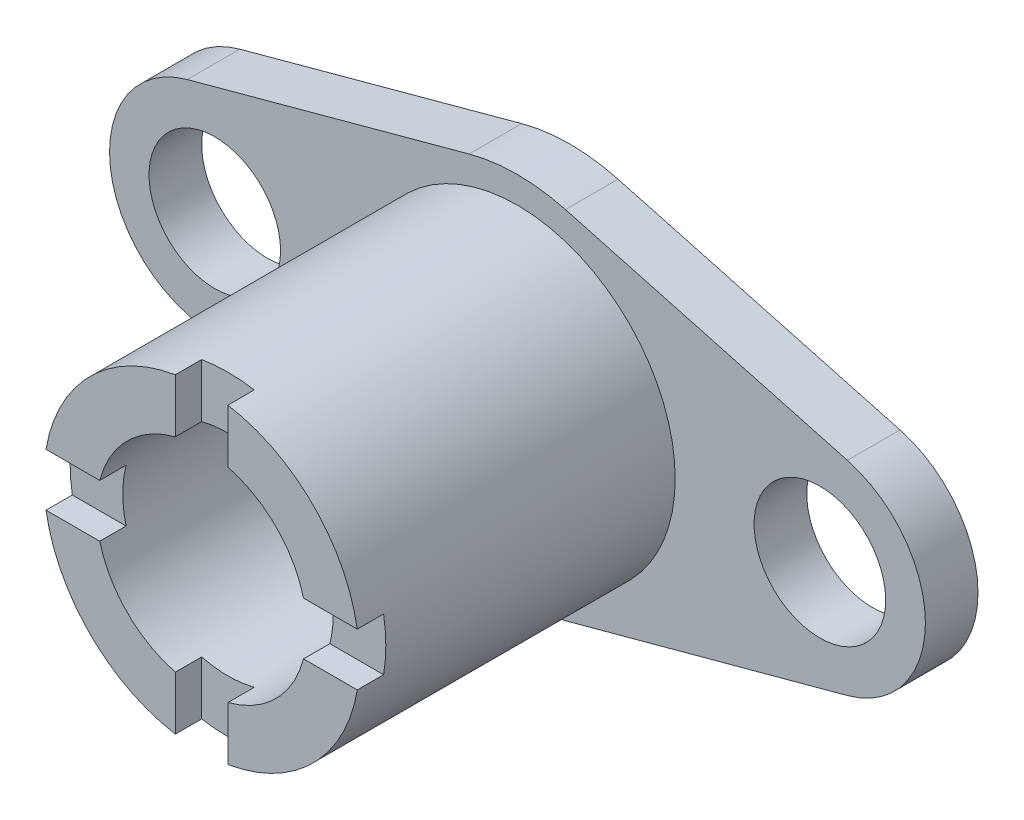
ISO-10303-21;
HEADER;
FILE_DESCRIPTION(('STEP AP214'),'2;1');
FILE_NAME('part.step','',(''),(''),'','','');
FILE_SCHEMA(('AUTOMOTIVE_DESIGN { 1 0 10303 214 1 1 1 1 }'));
ENDSEC;
DATA;
#1=APPLICATION_CONTEXT('core data for automotive mechanical design processes');
#2=APPLICATION_PROTOCOL_DEFINITION('international standard','automotive_design',2000,#1);
#3=PRODUCT_CONTEXT('',#1,'mechanical');
#4=PRODUCT('Part','Part','',(#3));
#5=PRODUCT_RELATED_PRODUCT_CATEGORY('part','',(#4));
#6=PRODUCT_DEFINITION_FORMATION('','',#4);
#7=PRODUCT_DEFINITION_CONTEXT('part definition',#1,'design');
#8=PRODUCT_DEFINITION('design','',#6,#7);
#9=PRODUCT_DEFINITION_SHAPE('','',#8);
#10=(LENGTH_UNIT() NAMED_UNIT(*) SI_UNIT(.MILLI.,.METRE.));
#11=(NAMED_UNIT(*) PLANE_ANGLE_UNIT() SI_UNIT($,.RADIAN.));
#12=(NAMED_UNIT(*) SI_UNIT($,.STERADIAN.) SOLID_ANGLE_UNIT());
#13=UNCERTAINTY_MEASURE_WITH_UNIT(LENGTH_MEASURE(1.E-05),#10,'distance_accuracy_value','');
#14=(GEOMETRIC_REPRESENTATION_CONTEXT(3) GLOBAL_UNCERTAINTY_ASSIGNED_CONTEXT((#13)) GLOBAL_UNIT_ASSIGNED_CONTEXT((#10,
#11,#12)) REPRESENTATION_CONTEXT('',''));
#15=CARTESIAN_POINT('',(0.,0.,0.));
#16=DIRECTION('',(0.,0.,1.));
#17=DIRECTION('',(1.,0.,0.));
#18=AXIS2_PLACEMENT_3D('',#15,#16,#17);
#19=CARTESIAN_POINT('',(0.,0.,70.));
#20=DIRECTION('',(0.,0.,-1.));
#21=DIRECTION('',(-1.,0.,0.));
#22=AXIS2_PLACEMENT_3D('',#19,#20,#21);
#23=CYLINDRICAL_SURFACE('',#22,30.);
#24=CARTESIAN_POINT('',(0.,0.,70.));
#25=DIRECTION('',(0.,0.,1.));
#26=DIRECTION('',(1.,0.,0.));
#27=AXIS2_PLACEMENT_3D('',#24,#25,#26);
#28=CIRCLE('',#27,30.);
#29=CARTESIAN_POINT('',(-29.5803989154981,-5.,70.));
#30=VERTEX_POINT('',#29);
#31=CARTESIAN_POINT('',(-5.,-29.5803989154981,70.));
#32=VERTEX_POINT('',#31);
#33=EDGE_CURVE('E751',#30,#32,#28,.T.);
#34=ORIENTED_EDGE('',*,*,#33,.F.);
#35=DIRECTION('',(0.,0.,1.));
#36=VECTOR('',#35,1.);
#37=CARTESIAN_POINT('',(-29.5803989154981,-5.,65.));
#38=LINE('',#37,#36);
#39=CARTESIAN_POINT('',(-29.5803989154981,-5.,65.));
#40=VERTEX_POINT('',#39);
#41=EDGE_CURVE('E233',#40,#30,#38,.T.);
#42=ORIENTED_EDGE('',*,*,#41,.F.);
#43=CARTESIAN_POINT('',(0.,0.,65.));
#44=DIRECTION('',(0.,0.,1.));
#45=DIRECTION('',(1.,0.,0.));
#46=AXIS2_PLACEMENT_3D('',#43,#44,#45);
#47=CIRCLE('',#46,30.);
#48=CARTESIAN_POINT('',(-29.5803989154981,5.,65.));
#49=VERTEX_POINT('',#48);
#50=EDGE_CURVE('E216',#49,#40,#47,.T.);
#51=ORIENTED_EDGE('',*,*,#50,.F.);
#52=DIRECTION('',(0.,0.,1.));
#53=VECTOR('',#52,1.);
#54=CARTESIAN_POINT('',(-29.5803989154981,5.,65.));
#55=LINE('',#54,#53);
#56=CARTESIAN_POINT('',(-29.5803989154981,5.,70.));
#57=VERTEX_POINT('',#56);
#58=EDGE_CURVE('E211',#49,#57,#55,.T.);
#59=ORIENTED_EDGE('',*,*,#58,.T.);
#60=CARTESIAN_POINT('',(-5.,29.5803989154981,70.));
#61=VERTEX_POINT('',#60);
#62=EDGE_CURVE('E324',#61,#57,#28,.T.);
#63=ORIENTED_EDGE('',*,*,#62,.F.);
#64=DIRECTION('',(0.,0.,1.));
#65=VECTOR('',#64,1.);
#66=CARTESIAN_POINT('',(-5.,29.5803989154981,65.));
#67=LINE('',#66,#65);
#68=CARTESIAN_POINT('',(-5.,29.5803989154981,65.));
#69=VERTEX_POINT('',#68);
#70=EDGE_CURVE('E257',#69,#61,#67,.T.);
#71=ORIENTED_EDGE('',*,*,#70,.F.);
#72=CARTESIAN_POINT('',(0.,0.,65.));
#73=DIRECTION('',(0.,0.,1.));
#74=DIRECTION('',(1.,0.,0.));
#75=AXIS2_PLACEMENT_3D('',#72,#73,#74);
#76=CIRCLE('',#75,30.);
#77=CARTESIAN_POINT('',(5.,29.5803989154981,65.));
#78=VERTEX_POINT('',#77);
#79=EDGE_CURVE('E238',#78,#69,#76,.T.);
#80=ORIENTED_EDGE('',*,*,#79,.F.);
#81=DIRECTION('',(0.,0.,1.));
#82=VECTOR('',#81,1.);
#83=CARTESIAN_POINT('',(5.,29.5803989154981,65.));
#84=LINE('',#83,#82);
#85=CARTESIAN_POINT('',(5.,29.5803989154981,70.));
#86=VERTEX_POINT('',#85);
#87=EDGE_CURVE('E242',#78,#86,#84,.T.);
#88=ORIENTED_EDGE('',*,*,#87,.T.);
#89=CARTESIAN_POINT('',(29.5803989154981,5.,70.));
#90=VERTEX_POINT('',#89);
#91=EDGE_CURVE('E316',#90,#86,#28,.T.);
#92=ORIENTED_EDGE('',*,*,#91,.F.);
#93=DIRECTION('',(0.,0.,1.));
#94=VECTOR('',#93,1.);
#95=CARTESIAN_POINT('',(29.5803989154981,5.,65.));
#96=LINE('',#95,#94);
#97=CARTESIAN_POINT('',(29.5803989154981,5.,65.));
#98=VERTEX_POINT('',#97);
#99=EDGE_CURVE('E310',#98,#90,#96,.T.);
#100=ORIENTED_EDGE('',*,*,#99,.F.);
#101=CARTESIAN_POINT('',(0.,0.,65.));
#102=DIRECTION('',(0.,0.,1.));
#103=DIRECTION('',(1.,0.,0.));
#104=AXIS2_PLACEMENT_3D('',#101,#102,#103);
#105=CIRCLE('',#104,30.);
#106=CARTESIAN_POINT('',(29.5803989154981,-5.,65.));
#107=VERTEX_POINT('',#106);
#108=EDGE_CURVE('E290',#107,#98,#105,.T.);
#109=ORIENTED_EDGE('',*,*,#108,.F.);
#110=DIRECTION('',(0.,0.,1.));
#111=VECTOR('',#110,1.);
#112=CARTESIAN_POINT('',(29.5803989154981,-5.,65.));
#113=LINE('',#112,#111);
#114=CARTESIAN_POINT('',(29.5803989154981,-5.,70.));
#115=VERTEX_POINT('',#114);
#116=EDGE_CURVE('E298',#107,#115,#113,.T.);
#117=ORIENTED_EDGE('',*,*,#116,.T.);
#118=CARTESIAN_POINT('',(5.,-29.5803989154981,70.));
#119=VERTEX_POINT('',#118);
#120=EDGE_CURVE('E321',#119,#115,#28,.T.);
#121=ORIENTED_EDGE('',*,*,#120,.F.);
#122=DIRECTION('',(0.,0.,1.));
#123=VECTOR('',#122,1.);
#124=CARTESIAN_POINT('',(5.,-29.5803989154981,65.));
#125=LINE('',#124,#123);
#126=CARTESIAN_POINT('',(5.,-29.5803989154981,65.));
#127=VERTEX_POINT('',#126);
#128=EDGE_CURVE('E272',#127,#119,#125,.T.);
#129=ORIENTED_EDGE('',*,*,#128,.F.);
#130=CARTESIAN_POINT('',(0.,0.,65.));
#131=DIRECTION('',(0.,0.,1.));
#132=DIRECTION('',(1.,0.,0.));
#133=AXIS2_PLACEMENT_3D('',#130,#131,#132);
#134=CIRCLE('',#133,30.);
#135=CARTESIAN_POINT('',(-5.,-29.5803989154981,65.));
#136=VERTEX_POINT('',#135);
#137=EDGE_CURVE('E258',#136,#127,#134,.T.);
#138=ORIENTED_EDGE('',*,*,#137,.F.);
#139=DIRECTION('',(0.,0.,1.));
#140=VECTOR('',#139,1.);
#141=CARTESIAN_POINT('',(-5.,-29.5803989154981,65.));
#142=LINE('',#141,#140);
#143=EDGE_CURVE('E247',#136,#32,#142,.T.);
#144=ORIENTED_EDGE('',*,*,#143,.T.);
#145=EDGE_LOOP('',(#34,#42,#51,#59,#63,#71,#80,#88,#92,#100,#109,#117,#121,#129,#138,#144));
#146=FACE_BOUND('',#145,.T.);
#147=CARTESIAN_POINT('',(0.,0.,10.));
#148=DIRECTION('',(0.,0.,1.));
#149=DIRECTION('',(1.,0.,0.));
#150=AXIS2_PLACEMENT_3D('',#147,#148,#149);
#151=CIRCLE('',#150,30.);
#152=CARTESIAN_POINT('',(30.,0.,10.));
#153=VERTEX_POINT('',#152);
#154=EDGE_CURVE('E313',#153,#153,#151,.T.);
#155=ORIENTED_EDGE('',*,*,#154,.T.);
#156=EDGE_LOOP('',(#155));
#157=FACE_BOUND('',#156,.T.);
#158=ADVANCED_FACE('F50',(#146,#157),#23,.T.);
#159=CARTESIAN_POINT('',(0.,0.,70.));
#160=DIRECTION('',(0.,0.,1.));
#161=DIRECTION('',(1.,0.,0.));
#162=AXIS2_PLACEMENT_3D('',#159,#160,#161);
#163=PLANE('',#162);
#164=DIRECTION('',(1.,0.,0.));
#165=VECTOR('',#164,1.);
#166=CARTESIAN_POINT('',(0.,-5.,70.));
#167=LINE('',#166,#165);
#168=CARTESIAN_POINT('',(-19.3649167310371,-5.,70.));
#169=VERTEX_POINT('',#168);
#170=EDGE_CURVE('E224',#30,#169,#167,.T.);
#171=ORIENTED_EDGE('',*,*,#170,.F.);
#172=ORIENTED_EDGE('',*,*,#33,.T.);
#173=DIRECTION('',(0.,1.,0.));
#174=VECTOR('',#173,1.);
#175=CARTESIAN_POINT('',(-5.,0.,70.));
#176=LINE('',#175,#174);
#177=CARTESIAN_POINT('',(-5.,-19.3649167310371,70.));
#178=VERTEX_POINT('',#177);
#179=EDGE_CURVE('E263',#32,#178,#176,.T.);
#180=ORIENTED_EDGE('',*,*,#179,.T.);
#181=CARTESIAN_POINT('',(0.,0.,70.));
#182=DIRECTION('',(0.,0.,1.));
#183=DIRECTION('',(1.,0.,0.));
#184=AXIS2_PLACEMENT_3D('',#181,#182,#183);
#185=CIRCLE('',#184,20.);
#186=EDGE_CURVE('E752',#169,#178,#185,.T.);
#187=ORIENTED_EDGE('',*,*,#186,.F.);
#188=EDGE_LOOP('',(#171,#172,#180,#187));
#189=FACE_BOUND('',#188,.T.);
#190=ADVANCED_FACE('F429',(#189),#163,.T.);
#191=ORIENTED_EDGE('',*,*,#91,.T.);
#192=DIRECTION('',(0.,-1.,0.));
#193=VECTOR('',#192,1.);
#194=CARTESIAN_POINT('',(5.,0.,70.));
#195=LINE('',#194,#193);
#196=CARTESIAN_POINT('',(5.,19.3649167310371,70.));
#197=VERTEX_POINT('',#196);
#198=EDGE_CURVE('E244',#86,#197,#195,.T.);
#199=ORIENTED_EDGE('',*,*,#198,.T.);
#200=CARTESIAN_POINT('',(19.3649167310371,5.,70.));
#201=VERTEX_POINT('',#200);
#202=EDGE_CURVE('E314',#201,#197,#185,.T.);
#203=ORIENTED_EDGE('',*,*,#202,.F.);
#204=DIRECTION('',(1.,0.,0.));
#205=VECTOR('',#204,1.);
#206=CARTESIAN_POINT('',(0.,5.,70.));
#207=LINE('',#206,#205);
#208=EDGE_CURVE('E289',#201,#90,#207,.T.);
#209=ORIENTED_EDGE('',*,*,#208,.T.);
#210=EDGE_LOOP('',(#191,#199,#203,#209));
#211=FACE_BOUND('',#210,.T.);
#212=ADVANCED_FACE('F434',(#211),#163,.T.);
#213=DIRECTION('',(-1.,0.,0.));
#214=VECTOR('',#213,1.);
#215=CARTESIAN_POINT('',(0.,5.,70.));
#216=LINE('',#215,#214);
#217=CARTESIAN_POINT('',(-19.3649167310371,5.,70.));
#218=VERTEX_POINT('',#217);
#219=EDGE_CURVE('E254',#218,#57,#216,.T.);
#220=ORIENTED_EDGE('',*,*,#219,.F.);
#221=CARTESIAN_POINT('',(-5.,19.3649167310371,70.));
#222=VERTEX_POINT('',#221);
#223=EDGE_CURVE('E230',#222,#218,#185,.T.);
#224=ORIENTED_EDGE('',*,*,#223,.F.);
#225=DIRECTION('',(0.,1.,0.));
#226=VECTOR('',#225,1.);
#227=CARTESIAN_POINT('',(-5.,0.,70.));
#228=LINE('',#227,#226);
#229=EDGE_CURVE('E237',#222,#61,#228,.T.);
#230=ORIENTED_EDGE('',*,*,#229,.T.);
#231=ORIENTED_EDGE('',*,*,#62,.T.);
#232=EDGE_LOOP('',(#220,#224,#230,#231));
#233=FACE_BOUND('',#232,.T.);
#234=ADVANCED_FACE('F480',(#233),#163,.T.);
#235=DIRECTION('',(0.,1.,0.));
#236=VECTOR('',#235,1.);
#237=CARTESIAN_POINT('',(5.,0.,70.));
#238=LINE('',#237,#236);
#239=CARTESIAN_POINT('',(5.,-19.3649167310371,70.));
#240=VERTEX_POINT('',#239);
#241=EDGE_CURVE('E275',#119,#240,#238,.T.);
#242=ORIENTED_EDGE('',*,*,#241,.F.);
#243=ORIENTED_EDGE('',*,*,#120,.T.);
#244=DIRECTION('',(-1.,0.,0.));
#245=VECTOR('',#244,1.);
#246=CARTESIAN_POINT('',(0.,-5.,70.));
#247=LINE('',#246,#245);
#248=CARTESIAN_POINT('',(19.3649167310371,-5.,70.));
#249=VERTEX_POINT('',#248);
#250=EDGE_CURVE('E300',#115,#249,#247,.T.);
#251=ORIENTED_EDGE('',*,*,#250,.T.);
#252=EDGE_CURVE('E319',#240,#249,#185,.T.);
#253=ORIENTED_EDGE('',*,*,#252,.F.);
#254=EDGE_LOOP('',(#242,#243,#251,#253));
#255=FACE_BOUND('',#254,.T.);
#256=ADVANCED_FACE('F438',(#255),#163,.T.);
#257=CARTESIAN_POINT('',(0.,0.,0.));
#258=DIRECTION('',(0.,0.,1.));
#259=DIRECTION('',(1.,0.,0.));
#260=AXIS2_PLACEMENT_3D('',#257,#258,#259);
#261=CYLINDRICAL_SURFACE('',#260,20.);
#262=CARTESIAN_POINT('',(0.,0.,0.));
#263=DIRECTION('',(0.,0.,1.));
#264=DIRECTION('',(1.,0.,0.));
#265=AXIS2_PLACEMENT_3D('',#262,#263,#264);
#266=CIRCLE('',#265,20.);
#267=CARTESIAN_POINT('',(20.,0.,0.));
#268=VERTEX_POINT('',#267);
#269=EDGE_CURVE('E311',#268,#268,#266,.T.);
#270=ORIENTED_EDGE('',*,*,#269,.F.);
#271=EDGE_LOOP('',(#270));
#272=FACE_BOUND('',#271,.T.);
#273=CARTESIAN_POINT('',(0.,0.,65.));
#274=DIRECTION('',(0.,0.,1.));
#275=DIRECTION('',(1.,0.,0.));
#276=AXIS2_PLACEMENT_3D('',#273,#274,#275);
#277=CIRCLE('',#276,20.);
#278=CARTESIAN_POINT('',(-19.3649167310371,-5.,65.));
#279=VERTEX_POINT('',#278);
#280=CARTESIAN_POINT('',(-19.3649167310371,5.,65.));
#281=VERTEX_POINT('',#280);
#282=EDGE_CURVE('E217',#279,#281,#277,.F.);
#283=ORIENTED_EDGE('',*,*,#282,.F.);
#284=DIRECTION('',(0.,0.,1.));
#285=VECTOR('',#284,1.);
#286=CARTESIAN_POINT('',(-19.3649167310371,-5.,65.));
#287=LINE('',#286,#285);
#288=EDGE_CURVE('E746',#279,#169,#287,.T.);
#289=ORIENTED_EDGE('',*,*,#288,.T.);
#290=ORIENTED_EDGE('',*,*,#186,.T.);
#291=DIRECTION('',(0.,0.,1.));
#292=VECTOR('',#291,1.);
#293=CARTESIAN_POINT('',(-5.,-19.3649167310371,65.));
#294=LINE('',#293,#292);
#295=CARTESIAN_POINT('',(-5.,-19.3649167310371,65.));
#296=VERTEX_POINT('',#295);
#297=EDGE_CURVE('E276',#296,#178,#294,.T.);
#298=ORIENTED_EDGE('',*,*,#297,.F.);
#299=CARTESIAN_POINT('',(0.,0.,65.));
#300=DIRECTION('',(0.,0.,1.));
#301=DIRECTION('',(1.,0.,0.));
#302=AXIS2_PLACEMENT_3D('',#299,#300,#301);
#303=CIRCLE('',#302,20.);
#304=CARTESIAN_POINT('',(5.,-19.3649167310371,65.));
#305=VERTEX_POINT('',#304);
#306=EDGE_CURVE('E267',#305,#296,#303,.F.);
#307=ORIENTED_EDGE('',*,*,#306,.F.);
#308=DIRECTION('',(0.,0.,1.));
#309=VECTOR('',#308,1.);
#310=CARTESIAN_POINT('',(5.,-19.3649167310371,65.));
#311=LINE('',#310,#309);
#312=EDGE_CURVE('E281',#305,#240,#311,.T.);
#313=ORIENTED_EDGE('',*,*,#312,.T.);
#314=ORIENTED_EDGE('',*,*,#252,.T.);
#315=DIRECTION('',(0.,0.,1.));
#316=VECTOR('',#315,1.);
#317=CARTESIAN_POINT('',(19.3649167310371,-5.,65.));
#318=LINE('',#317,#316);
#319=CARTESIAN_POINT('',(19.3649167310371,-5.,65.));
#320=VERTEX_POINT('',#319);
#321=EDGE_CURVE('E274',#320,#249,#318,.T.);
#322=ORIENTED_EDGE('',*,*,#321,.F.);
#323=CARTESIAN_POINT('',(0.,0.,65.));
#324=DIRECTION('',(0.,0.,1.));
#325=DIRECTION('',(1.,0.,0.));
#326=AXIS2_PLACEMENT_3D('',#323,#324,#325);
#327=CIRCLE('',#326,20.);
#328=CARTESIAN_POINT('',(19.3649167310371,5.,65.));
#329=VERTEX_POINT('',#328);
#330=EDGE_CURVE('E291',#329,#320,#327,.F.);
#331=ORIENTED_EDGE('',*,*,#330,.F.);
#332=DIRECTION('',(0.,0.,1.));
#333=VECTOR('',#332,1.);
#334=CARTESIAN_POINT('',(19.3649167310371,5.,65.));
#335=LINE('',#334,#333);
#336=EDGE_CURVE('E302',#329,#201,#335,.T.);
#337=ORIENTED_EDGE('',*,*,#336,.T.);
#338=ORIENTED_EDGE('',*,*,#202,.T.);
#339=DIRECTION('',(0.,0.,1.));
#340=VECTOR('',#339,1.);
#341=CARTESIAN_POINT('',(5.,19.3649167310371,65.));
#342=LINE('',#341,#340);
#343=CARTESIAN_POINT('',(5.,19.3649167310371,65.));
#344=VERTEX_POINT('',#343);
#345=EDGE_CURVE('E252',#344,#197,#342,.T.);
#346=ORIENTED_EDGE('',*,*,#345,.F.);
#347=CARTESIAN_POINT('',(0.,0.,65.));
#348=DIRECTION('',(0.,0.,1.));
#349=DIRECTION('',(1.,0.,0.));
#350=AXIS2_PLACEMENT_3D('',#347,#348,#349);
#351=CIRCLE('',#350,20.);
#352=CARTESIAN_POINT('',(-5.,19.3649167310371,65.));
#353=VERTEX_POINT('',#352);
#354=EDGE_CURVE('E245',#353,#344,#351,.F.);
#355=ORIENTED_EDGE('',*,*,#354,.F.);
#356=DIRECTION('',(0.,0.,1.));
#357=VECTOR('',#356,1.);
#358=CARTESIAN_POINT('',(-5.,19.3649167310371,65.));
#359=LINE('',#358,#357);
#360=EDGE_CURVE('E251',#353,#222,#359,.T.);
#361=ORIENTED_EDGE('',*,*,#360,.T.);
#362=ORIENTED_EDGE('',*,*,#223,.T.);
#363=DIRECTION('',(0.,0.,1.));
#364=VECTOR('',#363,1.);
#365=CARTESIAN_POINT('',(-19.3649167310371,5.,65.));
#366=LINE('',#365,#364);
#367=EDGE_CURVE('E212',#281,#218,#366,.T.);
#368=ORIENTED_EDGE('',*,*,#367,.F.);
#369=EDGE_LOOP('',(#283,#289,#290,#298,#307,#313,#314,#322,#331,#337,#338,#346,#355,#361,#362,#368));
#370=FACE_BOUND('',#369,.T.);
#371=ADVANCED_FACE('F228',(#272,#370),#261,.F.);
#372=CARTESIAN_POINT('',(9.14377412867148,33.8372678939061,10.));
#373=DIRECTION('',(0.260870913766134,0.965373692593092,0.));
#374=DIRECTION('',(-0.965373692593092,0.260870913766134,0.));
#375=AXIS2_PLACEMENT_3D('',#372,#373,#374);
#376=PLANE('',#375);
#377=DIRECTION('',(0.965373692593092,-0.260870913766134,0.));
#378=VECTOR('',#377,1.);
#379=CARTESIAN_POINT('',(9.14377412867148,33.8372678939061,0.));
#380=LINE('',#379,#378);
#381=CARTESIAN_POINT('',(9.14377412867149,33.8372678939061,0.));
#382=VERTEX_POINT('',#381);
#383=CARTESIAN_POINT('',(62.7306901938438,19.3565876484347,0.));
#384=VERTEX_POINT('',#383);
#385=EDGE_CURVE('E325',#382,#384,#380,.T.);
#386=ORIENTED_EDGE('',*,*,#385,.F.);
#387=DIRECTION('',(0.,0.,-1.));
#388=VECTOR('',#387,1.);
#389=CARTESIAN_POINT('',(9.14377412867149,33.8372678939061,10.));
#390=LINE('',#389,#388);
#391=CARTESIAN_POINT('',(9.14377412867149,33.8372678939061,10.));
#392=VERTEX_POINT('',#391);
#393=EDGE_CURVE('E11',#392,#382,#390,.T.);
#394=ORIENTED_EDGE('',*,*,#393,.F.);
#395=DIRECTION('',(0.965373692593092,-0.260870913766134,0.));
#396=VECTOR('',#395,1.);
#397=CARTESIAN_POINT('',(9.14377412867148,33.8372678939061,10.));
#398=LINE('',#397,#396);
#399=CARTESIAN_POINT('',(62.7306901938438,19.3565876484347,10.));
#400=VERTEX_POINT('',#399);
#401=EDGE_CURVE('E327',#392,#400,#398,.T.);
#402=ORIENTED_EDGE('',*,*,#401,.T.);
#403=DIRECTION('',(0.,0.,-1.));
#404=VECTOR('',#403,1.);
#405=CARTESIAN_POINT('',(62.7306901938438,19.3565876484347,10.));
#406=LINE('',#405,#404);
#407=EDGE_CURVE('E346',#400,#384,#406,.T.);
#408=ORIENTED_EDGE('',*,*,#407,.T.);
#409=EDGE_LOOP('',(#386,#394,#402,#408));
#410=FACE_BOUND('',#409,.T.);
#411=ADVANCED_FACE('F47',(#410),#376,.T.);
#412=CARTESIAN_POINT('',(0.,0.,10.));
#413=DIRECTION('',(0.,0.,-1.));
#414=DIRECTION('',(-1.,0.,0.));
#415=AXIS2_PLACEMENT_3D('',#412,#413,#414);
#416=CYLINDRICAL_SURFACE('',#415,35.0509529662195);
#417=CARTESIAN_POINT('',(0.,0.,0.));
#418=DIRECTION('',(0.,0.,1.));
#419=DIRECTION('',(1.,0.,0.));
#420=AXIS2_PLACEMENT_3D('',#417,#418,#419);
#421=CIRCLE('',#420,35.0509529662195);
#422=CARTESIAN_POINT('',(-9.17488842943839,33.8288445878291,0.));
#423=VERTEX_POINT('',#422);
#424=EDGE_CURVE('E348',#382,#423,#421,.T.);
#425=ORIENTED_EDGE('',*,*,#424,.T.);
#426=DIRECTION('',(0.,0.,-1.));
#427=VECTOR('',#426,1.);
#428=CARTESIAN_POINT('',(-9.17488842943839,33.8288445878291,10.));
#429=LINE('',#428,#427);
#430=CARTESIAN_POINT('',(-9.17488842943839,33.8288445878291,10.));
#431=VERTEX_POINT('',#430);
#432=EDGE_CURVE('E54',#431,#423,#429,.T.);
#433=ORIENTED_EDGE('',*,*,#432,.F.);
#434=CARTESIAN_POINT('',(0.,0.,10.));
#435=DIRECTION('',(0.,0.,1.));
#436=DIRECTION('',(1.,0.,0.));
#437=AXIS2_PLACEMENT_3D('',#434,#435,#436);
#438=CIRCLE('',#437,35.0509529662195);
#439=EDGE_CURVE('E330',#392,#431,#438,.T.);
#440=ORIENTED_EDGE('',*,*,#439,.F.);
#441=ORIENTED_EDGE('',*,*,#393,.T.);
#442=EDGE_LOOP('',(#425,#433,#440,#441));
#443=FACE_BOUND('',#442,.T.);
#444=ADVANCED_FACE('F390',(#443),#416,.T.);
#445=CARTESIAN_POINT('',(-9.1748884294384,33.8288445878291,10.));
#446=DIRECTION('',(-0.26175860149311,0.965133376557029,0.));
#447=DIRECTION('',(-0.965133376557029,-0.26175860149311,0.));
#448=AXIS2_PLACEMENT_3D('',#445,#446,#447);
#449=PLANE('',#448);
#450=DIRECTION('',(0.965133376557029,0.26175860149311,0.));
#451=VECTOR('',#450,1.);
#452=CARTESIAN_POINT('',(-9.1748884294384,33.8288445878291,0.));
#453=LINE('',#452,#451);
#454=CARTESIAN_POINT('',(-62.7351284157398,19.3025067209703,0.));
#455=VERTEX_POINT('',#454);
#456=EDGE_CURVE('E355',#455,#423,#453,.T.);
#457=ORIENTED_EDGE('',*,*,#456,.F.);
#458=DIRECTION('',(0.,0.,-1.));
#459=VECTOR('',#458,1.);
#460=CARTESIAN_POINT('',(-62.7351284157398,19.3025067209703,10.));
#461=LINE('',#460,#459);
#462=CARTESIAN_POINT('',(-62.7351284157398,19.3025067209703,10.));
#463=VERTEX_POINT('',#462);
#464=EDGE_CURVE('E377',#463,#455,#461,.T.);
#465=ORIENTED_EDGE('',*,*,#464,.F.);
#466=DIRECTION('',(0.965133376557029,0.26175860149311,0.));
#467=VECTOR('',#466,1.);
#468=CARTESIAN_POINT('',(-9.1748884294384,33.8288445878291,10.));
#469=LINE('',#468,#467);
#470=EDGE_CURVE('E334',#463,#431,#469,.T.);
#471=ORIENTED_EDGE('',*,*,#470,.T.);
#472=ORIENTED_EDGE('',*,*,#432,.T.);
#473=EDGE_LOOP('',(#457,#465,#471,#472));
#474=FACE_BOUND('',#473,.T.);
#475=ADVANCED_FACE('F385',(#474),#449,.T.);
#476=CARTESIAN_POINT('',(-57.5,0.,10.));
#477=DIRECTION('',(0.,0.,-1.));
#478=DIRECTION('',(-1.,0.,0.));
#479=AXIS2_PLACEMENT_3D('',#476,#477,#478);
#480=CYLINDRICAL_SURFACE('',#479,19.9998333803657);
#481=CARTESIAN_POINT('',(-57.5,0.,0.));
#482=DIRECTION('',(0.,0.,1.));
#483=DIRECTION('',(1.,0.,0.));
#484=AXIS2_PLACEMENT_3D('',#481,#482,#483);
#485=CIRCLE('',#484,19.9998333803657);
#486=CARTESIAN_POINT('',(-62.7351284157398,-19.3025067209703,0.));
#487=VERTEX_POINT('',#486);
#488=EDGE_CURVE('E353',#455,#487,#485,.T.);
#489=ORIENTED_EDGE('',*,*,#488,.T.);
#490=DIRECTION('',(0.,0.,-1.));
#491=VECTOR('',#490,1.);
#492=CARTESIAN_POINT('',(-62.7351284157398,-19.3025067209703,10.));
#493=LINE('',#492,#491);
#494=CARTESIAN_POINT('',(-62.7351284157398,-19.3025067209703,10.));
#495=VERTEX_POINT('',#494);
#496=EDGE_CURVE('E374',#495,#487,#493,.T.);
#497=ORIENTED_EDGE('',*,*,#496,.F.);
#498=CARTESIAN_POINT('',(-57.5,0.,10.));
#499=DIRECTION('',(0.,0.,1.));
#500=DIRECTION('',(1.,0.,0.));
#501=AXIS2_PLACEMENT_3D('',#498,#499,#500);
#502=CIRCLE('',#501,19.9998333803657);
#503=EDGE_CURVE('E337',#463,#495,#502,.T.);
#504=ORIENTED_EDGE('',*,*,#503,.F.);
#505=ORIENTED_EDGE('',*,*,#464,.T.);
#506=EDGE_LOOP('',(#489,#497,#504,#505));
#507=FACE_BOUND('',#506,.T.);
#508=ADVANCED_FACE('F397',(#507),#480,.T.);
#509=CARTESIAN_POINT('',(-9.17488842943839,-33.8288445878291,10.));
#510=DIRECTION('',(0.26175860149311,0.965133376557029,0.));
#511=DIRECTION('',(-0.965133376557029,0.26175860149311,0.));
#512=AXIS2_PLACEMENT_3D('',#509,#510,#511);
#513=PLANE('',#512);
#514=DIRECTION('',(0.965133376557029,-0.26175860149311,0.));
#515=VECTOR('',#514,1.);
#516=CARTESIAN_POINT('',(-9.17488842943839,-33.8288445878291,0.));
#517=LINE('',#516,#515);
#518=CARTESIAN_POINT('',(-9.17488842943839,-33.8288445878291,0.));
#519=VERTEX_POINT('',#518);
#520=EDGE_CURVE('E357',#487,#519,#517,.T.);
#521=ORIENTED_EDGE('',*,*,#520,.T.);
#522=DIRECTION('',(0.,0.,-1.));
#523=VECTOR('',#522,1.);
#524=CARTESIAN_POINT('',(-9.17488842943839,-33.8288445878291,10.));
#525=LINE('',#524,#523);
#526=CARTESIAN_POINT('',(-9.17488842943839,-33.8288445878291,10.));
#527=VERTEX_POINT('',#526);
#528=EDGE_CURVE('E375',#527,#519,#525,.T.);
#529=ORIENTED_EDGE('',*,*,#528,.F.);
#530=DIRECTION('',(0.965133376557029,-0.26175860149311,0.));
#531=VECTOR('',#530,1.);
#532=CARTESIAN_POINT('',(-9.17488842943839,-33.8288445878291,10.));
#533=LINE('',#532,#531);
#534=EDGE_CURVE('E336',#495,#527,#533,.T.);
#535=ORIENTED_EDGE('',*,*,#534,.F.);
#536=ORIENTED_EDGE('',*,*,#496,.T.);
#537=EDGE_LOOP('',(#521,#529,#535,#536));
#538=FACE_BOUND('',#537,.T.);
#539=ADVANCED_FACE('F398',(#538),#513,.F.);
#540=CARTESIAN_POINT('',(0.,0.,10.));
#541=DIRECTION('',(0.,0.,-1.));
#542=DIRECTION('',(-1.,0.,0.));
#543=AXIS2_PLACEMENT_3D('',#540,#541,#542);
#544=CYLINDRICAL_SURFACE('',#543,35.0509529662195);
#545=CARTESIAN_POINT('',(0.,0.,0.));
#546=DIRECTION('',(0.,0.,1.));
#547=DIRECTION('',(1.,0.,0.));
#548=AXIS2_PLACEMENT_3D('',#545,#546,#547);
#549=CIRCLE('',#548,35.0509529662195);
#550=CARTESIAN_POINT('',(9.14377412867149,-33.8372678939061,0.));
#551=VERTEX_POINT('',#550);
#552=EDGE_CURVE('E360',#519,#551,#549,.T.);
#553=ORIENTED_EDGE('',*,*,#552,.T.);
#554=DIRECTION('',(0.,0.,-1.));
#555=VECTOR('',#554,1.);
#556=CARTESIAN_POINT('',(9.14377412867149,-33.8372678939061,10.));
#557=LINE('',#556,#555);
#558=CARTESIAN_POINT('',(9.14377412867149,-33.8372678939061,10.));
#559=VERTEX_POINT('',#558);
#560=EDGE_CURVE('E367',#559,#551,#557,.T.);
#561=ORIENTED_EDGE('',*,*,#560,.F.);
#562=CARTESIAN_POINT('',(0.,0.,10.));
#563=DIRECTION('',(0.,0.,1.));
#564=DIRECTION('',(1.,0.,0.));
#565=AXIS2_PLACEMENT_3D('',#562,#563,#564);
#566=CIRCLE('',#565,35.0509529662195);
#567=EDGE_CURVE('E338',#527,#559,#566,.T.);
#568=ORIENTED_EDGE('',*,*,#567,.F.);
#569=ORIENTED_EDGE('',*,*,#528,.T.);
#570=EDGE_LOOP('',(#553,#561,#568,#569));
#571=FACE_BOUND('',#570,.T.);
#572=ADVANCED_FACE('F416',(#571),#544,.T.);
#573=CARTESIAN_POINT('',(9.14377412867149,-33.8372678939061,10.));
#574=DIRECTION('',(-0.260870913766134,0.965373692593092,0.));
#575=DIRECTION('',(-0.965373692593092,-0.260870913766134,0.));
#576=AXIS2_PLACEMENT_3D('',#573,#574,#575);
#577=PLANE('',#576);
#578=DIRECTION('',(0.965373692593092,0.260870913766135,0.));
#579=VECTOR('',#578,1.);
#580=CARTESIAN_POINT('',(9.14377412867149,-33.8372678939061,0.));
#581=LINE('',#580,#579);
#582=CARTESIAN_POINT('',(62.7306901938437,-19.3565876484347,0.));
#583=VERTEX_POINT('',#582);
#584=EDGE_CURVE('E363',#551,#583,#581,.T.);
#585=ORIENTED_EDGE('',*,*,#584,.T.);
#586=DIRECTION('',(0.,0.,-1.));
#587=VECTOR('',#586,1.);
#588=CARTESIAN_POINT('',(62.7306901938437,-19.3565876484347,10.));
#589=LINE('',#588,#587);
#590=CARTESIAN_POINT('',(62.7306901938437,-19.3565876484347,10.));
#591=VERTEX_POINT('',#590);
#592=EDGE_CURVE('E366',#591,#583,#589,.T.);
#593=ORIENTED_EDGE('',*,*,#592,.F.);
#594=DIRECTION('',(0.965373692593092,0.260870913766135,0.));
#595=VECTOR('',#594,1.);
#596=CARTESIAN_POINT('',(9.14377412867149,-33.8372678939061,10.));
#597=LINE('',#596,#595);
#598=EDGE_CURVE('E345',#559,#591,#597,.T.);
#599=ORIENTED_EDGE('',*,*,#598,.F.);
#600=ORIENTED_EDGE('',*,*,#560,.T.);
#601=EDGE_LOOP('',(#585,#593,#599,#600));
#602=FACE_BOUND('',#601,.T.);
#603=ADVANCED_FACE('F420',(#602),#577,.F.);
#604=CARTESIAN_POINT('',(57.5,0.,10.));
#605=DIRECTION('',(0.,0.,-1.));
#606=DIRECTION('',(-1.,0.,0.));
#607=AXIS2_PLACEMENT_3D('',#604,#605,#606);
#608=CYLINDRICAL_SURFACE('',#607,20.0508754246668);
#609=CARTESIAN_POINT('',(57.5,0.,0.));
#610=DIRECTION('',(0.,0.,1.));
#611=DIRECTION('',(1.,0.,0.));
#612=AXIS2_PLACEMENT_3D('',#609,#610,#611);
#613=CIRCLE('',#612,20.0508754246668);
#614=EDGE_CURVE('E332',#583,#384,#613,.T.);
#615=ORIENTED_EDGE('',*,*,#614,.T.);
#616=ORIENTED_EDGE('',*,*,#407,.F.);
#617=CARTESIAN_POINT('',(57.5,0.,10.));
#618=DIRECTION('',(0.,0.,1.));
#619=DIRECTION('',(1.,0.,0.));
#620=AXIS2_PLACEMENT_3D('',#617,#618,#619);
#621=CIRCLE('',#620,20.0508754246668);
#622=EDGE_CURVE('E341',#591,#400,#621,.T.);
#623=ORIENTED_EDGE('',*,*,#622,.F.);
#624=ORIENTED_EDGE('',*,*,#592,.T.);
#625=EDGE_LOOP('',(#615,#616,#623,#624));
#626=FACE_BOUND('',#625,.T.);
#627=ADVANCED_FACE('F414',(#626),#608,.T.);
#628=CARTESIAN_POINT('',(0.,0.,10.));
#629=DIRECTION('',(0.,0.,1.));
#630=DIRECTION('',(1.,0.,0.));
#631=AXIS2_PLACEMENT_3D('',#628,#629,#630);
#632=PLANE('',#631);
#633=CARTESIAN_POINT('',(-57.5,0.,10.));
#634=DIRECTION('',(0.,0.,1.));
#635=DIRECTION('',(1.,0.,0.));
#636=AXIS2_PLACEMENT_3D('',#633,#634,#635);
#637=CIRCLE('',#636,12.5);
#638=CARTESIAN_POINT('',(-45.,0.,10.));
#639=VERTEX_POINT('',#638);
#640=EDGE_CURVE('E733',#639,#639,#637,.T.);
#641=ORIENTED_EDGE('',*,*,#640,.F.);
#642=EDGE_LOOP('',(#641));
#643=FACE_BOUND('',#642,.T.);
#644=CARTESIAN_POINT('',(57.5,0.,10.));
#645=DIRECTION('',(0.,0.,1.));
#646=DIRECTION('',(1.,0.,0.));
#647=AXIS2_PLACEMENT_3D('',#644,#645,#646);
#648=CIRCLE('',#647,12.5);
#649=CARTESIAN_POINT('',(70.,0.,10.));
#650=VERTEX_POINT('',#649);
#651=EDGE_CURVE('E740',#650,#650,#648,.T.);
#652=ORIENTED_EDGE('',*,*,#651,.F.);
#653=EDGE_LOOP('',(#652));
#654=FACE_BOUND('',#653,.T.);
#655=ORIENTED_EDGE('',*,*,#154,.F.);
#656=EDGE_LOOP('',(#655));
#657=FACE_BOUND('',#656,.T.);
#658=ORIENTED_EDGE('',*,*,#401,.F.);
#659=ORIENTED_EDGE('',*,*,#439,.T.);
#660=ORIENTED_EDGE('',*,*,#470,.F.);
#661=ORIENTED_EDGE('',*,*,#503,.T.);
#662=ORIENTED_EDGE('',*,*,#534,.T.);
#663=ORIENTED_EDGE('',*,*,#567,.T.);
#664=ORIENTED_EDGE('',*,*,#598,.T.);
#665=ORIENTED_EDGE('',*,*,#622,.T.);
#666=EDGE_LOOP('',(#658,#659,#660,#661,#662,#663,#664,#665));
#667=FACE_BOUND('',#666,.T.);
#668=ADVANCED_FACE('F403',(#643,#654,#657,#667),#632,.T.);
#669=CARTESIAN_POINT('',(0.,0.,0.));
#670=DIRECTION('',(0.,0.,1.));
#671=DIRECTION('',(1.,0.,0.));
#672=AXIS2_PLACEMENT_3D('',#669,#670,#671);
#673=PLANE('',#672);
#674=CARTESIAN_POINT('',(-57.5,0.,0.));
#675=DIRECTION('',(0.,0.,1.));
#676=DIRECTION('',(1.,0.,0.));
#677=AXIS2_PLACEMENT_3D('',#674,#675,#676);
#678=CIRCLE('',#677,12.5);
#679=CARTESIAN_POINT('',(-45.,0.,0.));
#680=VERTEX_POINT('',#679);
#681=EDGE_CURVE('E297',#680,#680,#678,.T.);
#682=ORIENTED_EDGE('',*,*,#681,.T.);
#683=EDGE_LOOP('',(#682));
#684=FACE_BOUND('',#683,.T.);
#685=CARTESIAN_POINT('',(57.5,0.,0.));
#686=DIRECTION('',(0.,0.,1.));
#687=DIRECTION('',(1.,0.,0.));
#688=AXIS2_PLACEMENT_3D('',#685,#686,#687);
#689=CIRCLE('',#688,12.5);
#690=CARTESIAN_POINT('',(70.,0.,0.));
#691=VERTEX_POINT('',#690);
#692=EDGE_CURVE('E736',#691,#691,#689,.T.);
#693=ORIENTED_EDGE('',*,*,#692,.T.);
#694=EDGE_LOOP('',(#693));
#695=FACE_BOUND('',#694,.T.);
#696=ORIENTED_EDGE('',*,*,#269,.T.);
#697=EDGE_LOOP('',(#696));
#698=FACE_BOUND('',#697,.T.);
#699=ORIENTED_EDGE('',*,*,#385,.T.);
#700=ORIENTED_EDGE('',*,*,#614,.F.);
#701=ORIENTED_EDGE('',*,*,#584,.F.);
#702=ORIENTED_EDGE('',*,*,#552,.F.);
#703=ORIENTED_EDGE('',*,*,#520,.F.);
#704=ORIENTED_EDGE('',*,*,#488,.F.);
#705=ORIENTED_EDGE('',*,*,#456,.T.);
#706=ORIENTED_EDGE('',*,*,#424,.F.);
#707=EDGE_LOOP('',(#699,#700,#701,#702,#703,#704,#705,#706));
#708=FACE_BOUND('',#707,.T.);
#709=ADVANCED_FACE('F391',(#684,#695,#698,#708),#673,.F.);
#710=CARTESIAN_POINT('',(0.,-5.,65.));
#711=DIRECTION('',(0.,1.,0.));
#712=DIRECTION('',(0.,0.,1.));
#713=AXIS2_PLACEMENT_3D('',#710,#711,#712);
#714=PLANE('',#713);
#715=ORIENTED_EDGE('',*,*,#250,.F.);
#716=ORIENTED_EDGE('',*,*,#116,.F.);
#717=DIRECTION('',(-1.,0.,0.));
#718=VECTOR('',#717,1.);
#719=CARTESIAN_POINT('',(0.,-5.,65.));
#720=LINE('',#719,#718);
#721=EDGE_CURVE('E285',#107,#320,#720,.T.);
#722=ORIENTED_EDGE('',*,*,#721,.T.);
#723=ORIENTED_EDGE('',*,*,#321,.T.);
#724=EDGE_LOOP('',(#715,#716,#722,#723));
#725=FACE_BOUND('',#724,.T.);
#726=ADVANCED_FACE('F449',(#725),#714,.T.);
#727=CARTESIAN_POINT('',(0.,5.,65.));
#728=DIRECTION('',(0.,-1.,0.));
#729=DIRECTION('',(0.,0.,-1.));
#730=AXIS2_PLACEMENT_3D('',#727,#728,#729);
#731=PLANE('',#730);
#732=ORIENTED_EDGE('',*,*,#208,.F.);
#733=ORIENTED_EDGE('',*,*,#336,.F.);
#734=DIRECTION('',(1.,0.,0.));
#735=VECTOR('',#734,1.);
#736=CARTESIAN_POINT('',(0.,5.,65.));
#737=LINE('',#736,#735);
#738=EDGE_CURVE('E293',#329,#98,#737,.T.);
#739=ORIENTED_EDGE('',*,*,#738,.T.);
#740=ORIENTED_EDGE('',*,*,#99,.T.);
#741=EDGE_LOOP('',(#732,#733,#739,#740));
#742=FACE_BOUND('',#741,.T.);
#743=ADVANCED_FACE('F521',(#742),#731,.T.);
#744=CARTESIAN_POINT('',(0.,0.,65.));
#745=DIRECTION('',(0.,0.,1.));
#746=DIRECTION('',(1.,0.,0.));
#747=AXIS2_PLACEMENT_3D('',#744,#745,#746);
#748=PLANE('',#747);
#749=ORIENTED_EDGE('',*,*,#721,.F.);
#750=ORIENTED_EDGE('',*,*,#108,.T.);
#751=ORIENTED_EDGE('',*,*,#738,.F.);
#752=ORIENTED_EDGE('',*,*,#330,.T.);
#753=EDGE_LOOP('',(#749,#750,#751,#752));
#754=FACE_BOUND('',#753,.T.);
#755=ADVANCED_FACE('F535',(#754),#748,.T.);
#756=CARTESIAN_POINT('',(-5.,0.,65.));
#757=DIRECTION('',(1.,0.,0.));
#758=DIRECTION('',(0.,0.,-1.));
#759=AXIS2_PLACEMENT_3D('',#756,#757,#758);
#760=PLANE('',#759);
#761=ORIENTED_EDGE('',*,*,#179,.F.);
#762=ORIENTED_EDGE('',*,*,#143,.F.);
#763=DIRECTION('',(0.,1.,0.));
#764=VECTOR('',#763,1.);
#765=CARTESIAN_POINT('',(-5.,0.,65.));
#766=LINE('',#765,#764);
#767=EDGE_CURVE('E266',#136,#296,#766,.T.);
#768=ORIENTED_EDGE('',*,*,#767,.T.);
#769=ORIENTED_EDGE('',*,*,#297,.T.);
#770=EDGE_LOOP('',(#761,#762,#768,#769));
#771=FACE_BOUND('',#770,.T.);
#772=ADVANCED_FACE('F545',(#771),#760,.T.);
#773=CARTESIAN_POINT('',(5.,0.,65.));
#774=DIRECTION('',(1.,0.,0.));
#775=DIRECTION('',(0.,0.,-1.));
#776=AXIS2_PLACEMENT_3D('',#773,#774,#775);
#777=PLANE('',#776);
#778=ORIENTED_EDGE('',*,*,#241,.T.);
#779=ORIENTED_EDGE('',*,*,#312,.F.);
#780=DIRECTION('',(0.,1.,0.));
#781=VECTOR('',#780,1.);
#782=CARTESIAN_POINT('',(5.,0.,65.));
#783=LINE('',#782,#781);
#784=EDGE_CURVE('E264',#127,#305,#783,.T.);
#785=ORIENTED_EDGE('',*,*,#784,.F.);
#786=ORIENTED_EDGE('',*,*,#128,.T.);
#787=EDGE_LOOP('',(#778,#779,#785,#786));
#788=FACE_BOUND('',#787,.T.);
#789=ADVANCED_FACE('F558',(#788),#777,.F.);
#790=CARTESIAN_POINT('',(0.,0.,65.));
#791=DIRECTION('',(0.,0.,1.));
#792=DIRECTION('',(1.,0.,0.));
#793=AXIS2_PLACEMENT_3D('',#790,#791,#792);
#794=PLANE('',#793);
#795=ORIENTED_EDGE('',*,*,#137,.T.);
#796=ORIENTED_EDGE('',*,*,#784,.T.);
#797=ORIENTED_EDGE('',*,*,#306,.T.);
#798=ORIENTED_EDGE('',*,*,#767,.F.);
#799=EDGE_LOOP('',(#795,#796,#797,#798));
#800=FACE_BOUND('',#799,.T.);
#801=ADVANCED_FACE('F568',(#800),#794,.T.);
#802=CARTESIAN_POINT('',(5.,0.,65.));
#803=DIRECTION('',(-1.,0.,0.));
#804=DIRECTION('',(0.,0.,1.));
#805=AXIS2_PLACEMENT_3D('',#802,#803,#804);
#806=PLANE('',#805);
#807=ORIENTED_EDGE('',*,*,#198,.F.);
#808=ORIENTED_EDGE('',*,*,#87,.F.);
#809=DIRECTION('',(0.,-1.,0.));
#810=VECTOR('',#809,1.);
#811=CARTESIAN_POINT('',(5.,0.,65.));
#812=LINE('',#811,#810);
#813=EDGE_CURVE('E236',#78,#344,#812,.T.);
#814=ORIENTED_EDGE('',*,*,#813,.T.);
#815=ORIENTED_EDGE('',*,*,#345,.T.);
#816=EDGE_LOOP('',(#807,#808,#814,#815));
#817=FACE_BOUND('',#816,.T.);
#818=ADVANCED_FACE('F582',(#817),#806,.T.);
#819=CARTESIAN_POINT('',(-5.,0.,65.));
#820=DIRECTION('',(1.,0.,0.));
#821=DIRECTION('',(0.,0.,-1.));
#822=AXIS2_PLACEMENT_3D('',#819,#820,#821);
#823=PLANE('',#822);
#824=ORIENTED_EDGE('',*,*,#229,.F.);
#825=ORIENTED_EDGE('',*,*,#360,.F.);
#826=DIRECTION('',(0.,1.,0.));
#827=VECTOR('',#826,1.);
#828=CARTESIAN_POINT('',(-5.,0.,65.));
#829=LINE('',#828,#827);
#830=EDGE_CURVE('E70',#353,#69,#829,.T.);
#831=ORIENTED_EDGE('',*,*,#830,.T.);
#832=ORIENTED_EDGE('',*,*,#70,.T.);
#833=EDGE_LOOP('',(#824,#825,#831,#832));
#834=FACE_BOUND('',#833,.T.);
#835=ADVANCED_FACE('F595',(#834),#823,.T.);
#836=CARTESIAN_POINT('',(0.,0.,65.));
#837=DIRECTION('',(0.,0.,1.));
#838=DIRECTION('',(1.,0.,0.));
#839=AXIS2_PLACEMENT_3D('',#836,#837,#838);
#840=PLANE('',#839);
#841=ORIENTED_EDGE('',*,*,#813,.F.);
#842=ORIENTED_EDGE('',*,*,#79,.T.);
#843=ORIENTED_EDGE('',*,*,#830,.F.);
#844=ORIENTED_EDGE('',*,*,#354,.T.);
#845=EDGE_LOOP('',(#841,#842,#843,#844));
#846=FACE_BOUND('',#845,.T.);
#847=ADVANCED_FACE('F601',(#846),#840,.T.);
#848=CARTESIAN_POINT('',(0.,-5.,65.));
#849=DIRECTION('',(0.,-1.,0.));
#850=DIRECTION('',(0.,0.,-1.));
#851=AXIS2_PLACEMENT_3D('',#848,#849,#850);
#852=PLANE('',#851);
#853=ORIENTED_EDGE('',*,*,#170,.T.);
#854=ORIENTED_EDGE('',*,*,#288,.F.);
#855=DIRECTION('',(1.,0.,0.));
#856=VECTOR('',#855,1.);
#857=CARTESIAN_POINT('',(0.,-5.,65.));
#858=LINE('',#857,#856);
#859=EDGE_CURVE('E65',#40,#279,#858,.T.);
#860=ORIENTED_EDGE('',*,*,#859,.F.);
#861=ORIENTED_EDGE('',*,*,#41,.T.);
#862=EDGE_LOOP('',(#853,#854,#860,#861));
#863=FACE_BOUND('',#862,.T.);
#864=ADVANCED_FACE('F617',(#863),#852,.F.);
#865=CARTESIAN_POINT('',(0.,5.,65.));
#866=DIRECTION('',(0.,1.,0.));
#867=DIRECTION('',(0.,0.,1.));
#868=AXIS2_PLACEMENT_3D('',#865,#866,#867);
#869=PLANE('',#868);
#870=ORIENTED_EDGE('',*,*,#219,.T.);
#871=ORIENTED_EDGE('',*,*,#58,.F.);
#872=DIRECTION('',(-1.,0.,0.));
#873=VECTOR('',#872,1.);
#874=CARTESIAN_POINT('',(0.,5.,65.));
#875=LINE('',#874,#873);
#876=EDGE_CURVE('E206',#281,#49,#875,.T.);
#877=ORIENTED_EDGE('',*,*,#876,.F.);
#878=ORIENTED_EDGE('',*,*,#367,.T.);
#879=EDGE_LOOP('',(#870,#871,#877,#878));
#880=FACE_BOUND('',#879,.T.);
#881=ADVANCED_FACE('F209',(#880),#869,.F.);
#882=CARTESIAN_POINT('',(0.,0.,65.));
#883=DIRECTION('',(0.,0.,1.));
#884=DIRECTION('',(1.,0.,0.));
#885=AXIS2_PLACEMENT_3D('',#882,#883,#884);
#886=PLANE('',#885);
#887=ORIENTED_EDGE('',*,*,#282,.T.);
#888=ORIENTED_EDGE('',*,*,#876,.T.);
#889=ORIENTED_EDGE('',*,*,#50,.T.);
#890=ORIENTED_EDGE('',*,*,#859,.T.);
#891=EDGE_LOOP('',(#887,#888,#889,#890));
#892=FACE_BOUND('',#891,.T.);
#893=ADVANCED_FACE('F220',(#892),#886,.T.);
#894=CARTESIAN_POINT('',(57.5,0.,0.));
#895=DIRECTION('',(0.,0.,1.));
#896=DIRECTION('',(1.,0.,0.));
#897=AXIS2_PLACEMENT_3D('',#894,#895,#896);
#898=CYLINDRICAL_SURFACE('',#897,12.5);
#899=ORIENTED_EDGE('',*,*,#692,.F.);
#900=EDGE_LOOP('',(#899));
#901=FACE_BOUND('',#900,.T.);
#902=ORIENTED_EDGE('',*,*,#651,.T.);
#903=EDGE_LOOP('',(#902));
#904=FACE_BOUND('',#903,.T.);
#905=ADVANCED_FACE('F649',(#901,#904),#898,.F.);
#906=CARTESIAN_POINT('',(-57.5,0.,0.));
#907=DIRECTION('',(0.,0.,1.));
#908=DIRECTION('',(1.,0.,0.));
#909=AXIS2_PLACEMENT_3D('',#906,#907,#908);
#910=CYLINDRICAL_SURFACE('',#909,12.5);
#911=ORIENTED_EDGE('',*,*,#681,.F.);
#912=EDGE_LOOP('',(#911));
#913=FACE_BOUND('',#912,.T.);
#914=ORIENTED_EDGE('',*,*,#640,.T.);
#915=EDGE_LOOP('',(#914));
#916=FACE_BOUND('',#915,.T.);
#917=ADVANCED_FACE('F670',(#913,#916),#910,.F.);
#918=CLOSED_SHELL('',(#158,#190,#212,#234,#256,#371,#411,#444,#475,#508,#539,#572,#603,#627,
#668,#709,#726,#743,#755,#772,#789,#801,#818,#835,#847,#864,#881,#893,#905,#917));
#919=MANIFOLD_SOLID_BREP('B2',#918);
#920=ADVANCED_BREP_SHAPE_REPRESENTATION('',(#18,#919),#14);
#921=SHAPE_DEFINITION_REPRESENTATION(#9,#920);
ENDSEC;
END-ISO-10303-21;
